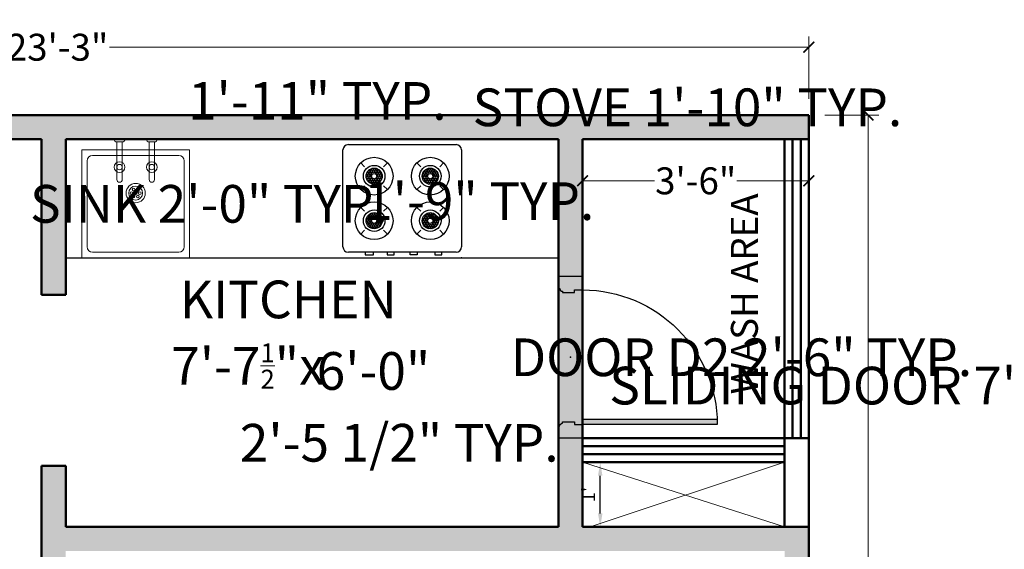
# Model space of a CAD drawing. Units: inches. Extents: x 4508 to 5907, y 877 to 1592.
# Tile 18 of 20: x 5383 to 5566, y 1494 to 1592. Entities that reach past the tile are written whole.
import ezdxf

# ---------------------------------------------------------------- set-up
doc = ezdxf.new("R2010")
doc.units = ezdxf.units.IN
doc.layers.get('DEFPOINTS').update_dxf_attribs({"color": 8})
for name, color, linetype, lineweight in [('A-ANNO-DIMS', 2, 'Continuous', 18), ('A-ANNO-TEXT', 7, 'Continuous', 25), ('A-DOOR', 4, 'Continuous', 25), ('A-FLOR-CASE', 30, 'Continuous', 25), ('A-FLOR-FIXT', 8, 'Continuous', 18), ('A-FLOR-SHFT', 8, 'Continuous', 18), ('A-WALL', 7, 'Continuous', 50), ('A-WALL-PATT', 8, 'Continuous', 13)]:
    doc.layers.add(name, color=color, linetype=linetype, lineweight=lineweight)
doc.layers.add('doors & windows', color=30, linetype='Continuous')
doc.layers.add('furniture', color=24, linetype='Continuous')
doc.styles.get("Standard").update_dxf_attribs({"font": 'arial.ttf'})
doc.dimstyles.new('details', dxfattribs={"dimtxt": 5, "dimasz": 2, "dimexe": 2, "dimexo": 3, "dimgap": 1, "dimtad": 0, "dimdec": 1, "dimzin": 0, "dimdsep": 46, "dimlunit": 4, "dimtxsty": 'Standard', "dimblk": 'ARCHTICK', "dimcen": 3, "dimclrd": 256, "dimclre": 256, "dimclrt": 256, "dimadec": 0, "dimazin": 0, "dimtfac": 0.5, "dimtdec": 1, "dimtofl": 0, "dimtmove": 0, "dimatfit": 3, "dimldrblk": 'CLOSEDBLANK', "dimfxl": 2, "dimtolj": 1, "dimtzin": 0, "dimlwd": -1, "dimlwe": -1, "dimarcsym": 0})
doc.dimstyles.new('ISO-25', dxfattribs={"dimtxt": 2.5, "dimasz": 2.5, "dimexe": 1.25, "dimexo": 0.625, "dimtad": 1, "dimdec": 0, "dimlunit": 4, "dimtxsty": 'Standard', "dimcen": 2.5, "dimadec": 0, "dimazin": 0, "dimtfac": 1, "dimtdec": 0, "dimtmove": 0, "dimatfit": 3, "dimfxl": 1, "dimarcsym": 0})
doc.dimstyles.new('text', dxfattribs={"dimtxt": 7, "dimasz": 0, "dimexe": 3, "dimexo": 3, "dimgap": 0, "dimtad": 1, "dimtih": 1, "dimtoh": 1, "dimzin": 3, "dimdsep": 46, "dimlunit": 4, "dimtxsty": 'Standard', "dimblk": 'CLOSEDBLANK', "dimcen": 3, "dimse1": 1, "dimse2": 1, "dimsd1": 1, "dimsd2": 1, "dimclrd": 256, "dimclre": 256, "dimclrt": 256, "dimadec": 0, "dimazin": 0, "dimtfac": 0.5, "dimtofl": 0, "dimtmove": 0, "dimatfit": 3, "dimfxl": 3, "dimtolj": 1, "dimtzin": 0, "dimlwd": -1, "dimlwe": -1, "dimarcsym": 0})

# ---------------------------------------------------------------- blocks, each defined once
blk = doc.blocks.new('*D78')
at = {"layer": 'DEFPOINTS', "color": 0, "transparency": 16777216}
for p in [(5391.9, 1545.16), (5483.4, 1536.45), (5483.4, 1523.93)]:
    blk.add_point(p, dxfattribs=at)
at = {"layer": 'A-ANNO-DIMS', "color": 0, "transparency": 16777216, "insert": (5425.76, 1533.92), "char_height": 7, "attachment_point": 5}
blk.add_mtext('\\A1;       KITCHEN\\P7\'-7{\\H0.5x;\\S1/2;}"x', dxfattribs=at)
blk = doc.blocks.new('_ClosedBlank')
at = {"color": 0, "lineweight": -2}
for p, q in [((-1, 0.167), (0, 0)), ((-1, 0.167), (-1, -0.167)), ((0, 0), (-1, -0.167))]:
    blk.add_line(p, q, dxfattribs=at)
blk = doc.blocks.new('*D79')
at = {"layer": 'DEFPOINTS', "color": 0, "transparency": 16777216}
for p in [(5431.17, 1570.2), (5449.06, 1570.2), (5421.9, 1498.2)]:
    blk.add_point(p, dxfattribs=at)
at = {"layer": 'A-ANNO-DIMS', "color": 0, "transparency": 16777216, "insert": (5449.06, 1527.16), "char_height": 7, "attachment_point": 5}
blk.add_mtext('\\A1;6\'-0"', dxfattribs=at)
blk = doc.blocks.new('stove')
at = {"layer": 'furniture'}
h = blk.add_hatch(dxfattribs=at)
h.set_pattern_fill('HEX', color=256, angle=180, style=0)
h.set_pattern_definition([(360, (22, 21.5), (1e-16, 0.2165064), [0.125, -0.25]), (120, (22, 21.5), (-0.1875, -0.1082532), [0.125, -0.25]), (60, (22.125, 21.5), (-0.1875, 0.1082532), [0.125, -0.25])])
h.paths.add_polyline_path([(5.36, 16.21, 1), (8.36, 16.21, 1)])
h.paths.add_polyline_path([(7.36, 16.21, -1), (6.36, 16.21, -1)], flags=16)
h = blk.add_hatch(dxfattribs=at)
h.set_pattern_fill('HEX', color=256, angle=180, style=0)
h.set_pattern_definition([(180, (2e-13, 21.5), (-1e-16, 0.2165064), [0.125, -0.25]), (60, (2e-13, 21.5), (0.1875, -0.1082532), [0.125, -0.25]), (120, (-0.125, 21.5), (0.1875, 0.1082532), [0.125, -0.25])])
h.paths.add_polyline_path([(13.64, 16.21, 1), (16.64, 16.21, 1)])
h.paths.add_polyline_path([(15.64, 16.21, -1), (14.64, 16.21, -1)], flags=16)
h = blk.add_hatch(dxfattribs=at)
h.set_pattern_fill('HEX', color=256, angle=180, style=0)
h.set_pattern_definition([(360, (22, 0.5), (-1e-16, -0.2165064), [0.125, -0.25]), (240, (22, 0.5), (-0.1875, 0.1082532), [0.125, -0.25]), (300, (22.125, 0.5), (-0.1875, -0.1082532), [0.125, -0.25])])
h.paths.add_polyline_path([(8.36, 5.79, 1), (5.36, 5.79, 1)])
h.paths.add_polyline_path([(6.36, 5.79, -1), (7.36, 5.79, -1)], flags=16)
h = blk.add_hatch(dxfattribs=at)
h.set_pattern_fill('HEX', color=256, angle=180, style=0)
h.set_pattern_definition([(180, (2e-13, 0.5), (1e-16, -0.2165064), [0.125, -0.25]), (300, (2e-13, 0.5), (0.1875, 0.1082532), [0.125, -0.25]), (240, (-0.125, 0.5), (0.1875, -0.1082532), [0.125, -0.25])])
h.paths.add_polyline_path([(16.64, 5.79, 1), (13.64, 5.79, 1)])
h.paths.add_polyline_path([(14.64, 5.79, -1), (15.64, 5.79, -1)], flags=16)
for p, q in [((2, 22), (20, 22)), ((1, 1), (1, 21)), ((21, 21), (21, 1)), ((4.39, 18.69), (5.1, 17.98)), ((8.63, 17.98), (9.34, 18.69)), ((13.37, 17.98), (12.66, 18.69)), ((17.61, 18.69), (16.9, 17.98)), ((1, 17.86), (0.5, 17.86)), ((0.5, 17.86), (0.5, 16.36)), ((0.5, 16.36), (1, 16.36)), ((0.5, 13.8), (0.5, 12.5)), ((1, 13.8), (0.5, 13.8)), ((4.39, 13.74), (5.1, 14.45)), ((8.63, 14.45), (9.34, 13.74)), ((13.37, 14.45), (12.66, 13.74)), ((17.61, 13.74), (16.9, 14.45)), ((0.5, 12.5), (1, 12.5)), ((0.5, 9.5), (1, 9.5)), ((0.5, 8.2), (0.5, 9.5)), ((1, 8.2), (0.5, 8.2)), ((4.39, 8.26), (5.1, 7.55)), ((8.63, 7.55), (9.34, 8.26)), ((13.37, 7.55), (12.66, 8.26)), ((17.61, 8.26), (16.9, 7.55)), ((0.5, 4.94), (0.5, 3.64)), ((1, 4.94), (0.5, 4.94)), ((4.39, 3.31), (5.1, 4.02)), ((8.63, 4.02), (9.34, 3.31)), ((13.37, 4.02), (12.66, 3.31)), ((17.61, 3.31), (16.9, 4.02)), ((0.5, 3.64), (1, 3.64)), ((20, 0), (2, 0))]:
    blk.add_line(p, q, dxfattribs=at)
for centre, radius in [((6.86, 16.21), 3.5), ((15.14, 16.21), 3.5), ((6.86, 16.21), 2), ((6.86, 16.21), 1.5), ((6.86, 16.21), 0.5), ((15.14, 16.21), 2), ((15.14, 16.21), 1.5), ((15.14, 16.21), 0.5), ((6.86, 5.79), 3.5), ((15.14, 5.79), 3.5), ((6.86, 5.79), 2), ((15.14, 5.79), 2), ((6.86, 5.79), 1.5), ((6.86, 5.79), 0.5), ((15.14, 5.79), 1.5), ((15.14, 5.79), 0.5)]:
    blk.add_circle(centre, radius, dxfattribs=at)
for centre, start, end in [((2, 21), 90, 180), ((20, 21), 0, 90), ((2, 1), 180, 270), ((20, 1), 270, 0)]:
    blk.add_arc(centre, 1, start, end, dxfattribs=at)
at = {"layer": 'furniture', "ltscale": 9}
blk.add_point((0, 0), dxfattribs=at)
blk = doc.blocks.new('sink')
for p, q in [((0, 0), (-24, 0)), ((0, 0), (0, 0)), ((-22, -3), (-2, -3)), ((-22, -23), (-22, -3)), ((-2, -3), (-2, -23)), ((-21, -21), (-21, -5)), ((-20, -4), (-4, -4)), ((-3, -5), (-3, -21)), ((0, -9), (0, -11)), ((-0.5, -9.5), (-7.5, -9.5)), ((-0.5, -10.5), (-7.5, -10.5)), ((-0.5, -9.5), (-0.5, -10.5)), ((-0.5, -15.5), (-7.5, -15.5)), ((-0.5, -15.5), (-0.5, -16.5)), ((0, -15), (0, -17)), ((-0.5, -16.5), (-7.5, -16.5)), ((-22, -23), (-2, -23)), ((-20, -22), (-4, -22))]:
    blk.add_line(p, q)
for centre, radius in [((-5.18, -10), 1), ((-5.18, -10), 0.5), ((-10, -13), 1.79), ((-10, -13), 1.29), ((-10.66, -12.62), 0.25), ((-10, -12.24), 0.25), ((-10, -13), 0.25), ((-9.34, -12.62), 0.25), ((-10.66, -13.38), 0.25), ((-10, -13.76), 0.25), ((-9.34, -13.38), 0.25), ((-5.18, -16), 1), ((-5.18, -16), 0.5)]:
    blk.add_circle(centre, radius)
for centre, radius, start, end in [((-20, -5), 1, 90, 180), ((-4, -5), 1, 0, 90), ((0.01, -9.51), 0.511, 91.1728, 178.8272), ((-7.5, -10), 0.5, 90, 270), ((0.01, -10.49), 0.511, 181.1728, 268.8272), ((-7.5, -16), 0.5, 90, 270), ((0.01, -15.51), 0.511, 91.1728, 178.8272), ((0.01, -16.49), 0.511, 181.1728, 268.8272), ((-20, -21), 1, 180, 270), ((-4, -21), 1, 270, 0)]:
    blk.add_arc(centre, radius, start, end)
blk = doc.blocks.new('*D80')
at = {"layer": 'A-ANNO-DIMS', "color": 0, "lineweight": -2, "transparency": 16777216}
for p, q in [((5488.53, 1510.2), (5492.43, 1510.2)), ((5491.18, 1500.7), (5491.18, 1507.7)), ((5488.53, 1498.2), (5492.43, 1498.2))]:
    blk.add_line(p, q, dxfattribs=at)
at = {"layer": 'A-ANNO-DIMS', "color": 0, "transparency": 16777216}
for points in [[(5490.76, 1507.7), (5491.59, 1507.7), (5491.18, 1510.2)], [(5490.76, 1500.7), (5491.59, 1500.7), (5491.18, 1498.2)]]:
    blk.add_solid(points, dxfattribs=at)
at = {"layer": 'DEFPOINTS', "color": 0, "transparency": 16777216}
for p in [(5487.9, 1510.2), (5491.18, 1510.2), (5487.9, 1498.2)]:
    blk.add_point(p, dxfattribs=at)
at = {"layer": 'A-ANNO-DIMS', "color": 0, "transparency": 16777216, "insert": (5489.3, 1504.2), "char_height": 2.5, "attachment_point": 5, "rotation": 90}
blk.add_mtext("1'", dxfattribs=at)
blk = doc.blocks.new('D2')
at = {"layer": 'doors & windows'}
h = blk.add_hatch(dxfattribs=at)
h.set_pattern_fill('DOTS', color=256, scale=2, angle=180, style=0)
h.set_pattern_definition([(180, (0, -4), (-0.0625, -0.125), [0, -0.125])])
h.paths.add_polyline_path([(2.5, 0), (3.5, 0), (3.5, 24.98, 0.010003), (2.5, 25)])
h = blk.add_hatch(dxfattribs=at)
h.set_pattern_fill('DOTS', color=256, scale=2, angle=180, style=0)
h.set_pattern_definition([(180, (0, 0), (-0.0625, -0.125), [0, -0.125])])
edge = h.paths.add_edge_path()
edge.add_line((27.5, 0), (27.5, -1.5))
edge.add_line((27.5, -1.5), (27, -1.5))
edge.add_line((27, -1.5), (27, -3.75))
edge.add_line((27, -3.75), (27.25, -3.75))
edge.add_arc((27.76, -3.74), 0.509, 181.0059, 268.9941)
edge.add_line((27.75, -4.25), (27.75, -4.5))
edge.add_line((27.75, -4.5), (30, -4.5))
edge.add_line((30, -4.5), (30, 0))
edge.add_line((30, 0), (27.5, 0))
edge = h.paths.add_edge_path()
edge.add_line((2.5, -1.5), (2.5, 0))
edge.add_line((2.5, 0), (0, 0))
edge.add_line((0, 0), (0, -4.5))
edge.add_line((0, -4.5), (2.25, -4.5))
edge.add_line((2.25, -4.5), (2.25, -4.25))
edge.add_arc((2.24, -3.74), 0.509, 271.0059, 358.9941)
edge.add_line((2.75, -3.75), (3, -3.75))
edge.add_line((3, -3.75), (3, -1.5))
edge.add_line((3, -1.5), (2.5, -1.5))
for p, q in [((0, 0), (0, -4.5)), ((30, 0), (30, -4.5))]:
    blk.add_line(p, q)
blk.add_lwpolyline([(3.5, 0), (3.5, 25), (2.5, 25), (2.5, 0)], close=True, dxfattribs=at)
for points in [[(3, -3.75), (3, -1.5), (2.5, -1.5), (2.5, 0), (0, 0)], [(27, -3.75), (27, -1.5), (27.5, -1.5), (27.5, 0), (30, 0)], [(0, -4.5), (2.25, -4.5)], [(30, -4.5), (27.75, -4.5)]]:
    blk.add_lwpolyline(points, dxfattribs=at)
for points in [[(2.25, -4.5), (2.25, -4.25, 0.403966), (2.75, -3.75), (3, -3.75)], [(27.75, -4.5), (27.75, -4.25, -0.403966), (27.25, -3.75), (27, -3.75)]]:
    blk.add_lwpolyline(points, format="xyb", dxfattribs=at)
at = {"layer": 'doors & windows', "ltscale": 6}
blk.add_arc((2.5, 0), 25, 0, 90, dxfattribs=at)
at = {"layer": 'doors & windows'}
blk.add_point((15, -2.25), dxfattribs=at)
blk = doc.blocks.new('_ArchTick')
at = {"color": 0, "linetype": 'ByBlock', "const_width": 0.15}
blk.add_lwpolyline([(-0.5, -0.5), (0.5, 0.5)], dxfattribs=at)
blk = doc.blocks.new('*D81')
at = {"layer": 'A-ANNO-DIMS', "color": 0, "transparency": 16777216}
for p, q in [((5487.9, 1567.2), (5487.9, 1560.48)), ((5529.9, 1567.2), (5529.9, 1560.48)), ((5487.9, 1562.48), (5501.26, 1562.48)), ((5529.9, 1562.48), (5516.55, 1562.48))]:
    blk.add_line(p, q, dxfattribs=at)
at = {"layer": 'DEFPOINTS', "color": 0, "transparency": 16777216}
for p in [(5487.9, 1570.2), (5529.9, 1570.2), (5529.9, 1562.48)]:
    blk.add_point(p, dxfattribs=at)
at = {"layer": 'A-ANNO-DIMS', "color": 0, "transparency": 16777216, "xscale": 2, "yscale": 2, "zscale": 2, "rotation": 180}
blk.add_blockref('_ArchTick', (5487.9, 1562.48), dxfattribs=at)
at = {"layer": 'A-ANNO-DIMS', "color": 0, "transparency": 16777216, "xscale": 2, "yscale": 2, "zscale": 2}
blk.add_blockref('_ArchTick', (5529.9, 1562.48), dxfattribs=at)
at = {"layer": 'A-ANNO-DIMS', "color": 0, "transparency": 16777216, "insert": (5508.9, 1562.48), "char_height": 5, "attachment_point": 5}
blk.add_mtext('\\A1;3\'-6"', dxfattribs=at)
blk = doc.blocks.new('*D82')
at = {"layer": 'DEFPOINTS', "color": 0, "transparency": 16777216}
for p in [(5255.4, 1510.81), (5387.4, 1507.41), (5387.4, 1493.7)]:
    blk.add_point(p, dxfattribs=at)
at = {"layer": 'A-ANNO-DIMS', "color": 0, "transparency": 16777216, "insert": (5317.71, 1516.81), "char_height": 7, "width": 116.2892, "attachment_point": 5}
blk.add_mtext('\\A1;       HALL\\P11\'-0"x', dxfattribs=at)
blk = doc.blocks.new('*D112')
at = {"layer": 'A-ANNO-DIMS', "color": 0, "transparency": 16777216}
for p, q in [((5250.9, 1577.7), (5250.9, 1589.3)), ((5529.9, 1577.7), (5529.9, 1589.3)), ((5250.9, 1587.3), (5380.77, 1587.3)), ((5529.9, 1587.3), (5400.03, 1587.3))]:
    blk.add_line(p, q, dxfattribs=at)
at = {"layer": 'DEFPOINTS', "color": 0, "transparency": 16777216}
for p in [(5529.9, 1587.3), (5250.9, 1574.7), (5529.9, 1574.7)]:
    blk.add_point(p, dxfattribs=at)
at = {"layer": 'A-ANNO-DIMS', "color": 0, "transparency": 16777216, "xscale": 2, "yscale": 2, "zscale": 2, "rotation": 180}
blk.add_blockref('_ArchTick', (5250.9, 1587.3), dxfattribs=at)
at = {"layer": 'A-ANNO-DIMS', "color": 0, "transparency": 16777216, "xscale": 2, "yscale": 2, "zscale": 2}
blk.add_blockref('_ArchTick', (5529.9, 1587.3), dxfattribs=at)
at = {"layer": 'A-ANNO-DIMS', "color": 0, "transparency": 16777216, "insert": (5390.4, 1587.3), "char_height": 5, "attachment_point": 5}
blk.add_mtext('\\A1;23\'-3"', dxfattribs=at)
blk = doc.blocks.new('*D113')
at = {"layer": 'A-ANNO-DIMS', "color": 0, "transparency": 16777216}
for p, q in [((5532.9, 1574.7), (5542.92, 1574.7)), ((5540.92, 1574.7), (5540.92, 1255.95)), ((5540.92, 926.7), (5540.92, 1245.46)), ((5532.9, 926.7), (5542.92, 926.7))]:
    blk.add_line(p, q, dxfattribs=at)
at = {"layer": 'DEFPOINTS', "color": 0, "transparency": 16777216}
for p in [(5529.9, 1574.7), (5540.92, 1574.7), (5529.9, 926.7)]:
    blk.add_point(p, dxfattribs=at)
at = {"layer": 'A-ANNO-DIMS', "color": 0, "transparency": 16777216, "xscale": 2, "yscale": 2, "zscale": 2}
for p, rotation in [((5540.92, 1574.7), 90), ((5540.92, 926.7), 270)]:
    blk.add_blockref('_ArchTick', p, dxfattribs=dict(at, rotation=rotation))
at = {"layer": 'A-ANNO-DIMS', "color": 0, "transparency": 16777216, "insert": (5540.92, 1250.7), "char_height": 5, "attachment_point": 5, "rotation": 90}
blk.add_mtext("\\A1;54'", dxfattribs=at)
blk = doc.blocks.new('*D146')
at = {"layer": 'DEFPOINTS', "color": 0, "transparency": 16777216}
for p in [(5512.9, 1544.7), (5517.4, 1544.7), (5512.9, 1514.7)]:
    blk.add_point(p, dxfattribs=at)
at = {"layer": 'A-ANNO-DIMS', "transparency": 16777216, "insert": (5517.4, 1529.7), "char_height": 7, "attachment_point": 5}
blk.add_mtext('\\A1;DOOR D2 2\'-6" TYP.', dxfattribs=at)
blk = doc.blocks.new('*D147')
at = {"layer": 'DEFPOINTS', "color": 0, "transparency": 16777216}
for p in [(5483.4, 1514.7), (5512.9, 1514.7), (5512.9, 1510.2)]:
    blk.add_point(p, dxfattribs=at)
at = {"layer": 'A-ANNO-DIMS', "transparency": 16777216, "insert": (5453.85, 1513.82), "char_height": 7, "attachment_point": 5}
blk.add_mtext('\\A1;2\'-5 1/2" TYP.', dxfattribs=at)
blk = doc.blocks.new('*D150')
at = {"layer": 'DEFPOINTS', "color": 0, "transparency": 16777216}
for p in [(5583.45, 1533.42), (5667.45, 1533.42), (5667.45, 1520.82)]:
    blk.add_point(p, dxfattribs=at)
at = {"layer": 'A-ANNO-DIMS', "transparency": 16777216, "insert": (5537.21, 1524.44), "char_height": 7, "attachment_point": 5}
blk.add_mtext('\\A1;SLIDING DOOR 7\'-0"', dxfattribs=at)
blk = doc.blocks.new('*D162')
at = {"layer": 'DEFPOINTS', "color": 0, "transparency": 16777216}
for p in [(5443.4, 1572.5), (5443.4, 1569.2), (5465.4, 1569.2)]:
    blk.add_point(p, dxfattribs=at)
at = {"layer": 'A-ANNO-DIMS', "transparency": 16777216, "insert": (5507.37, 1576.13), "char_height": 7, "attachment_point": 5}
blk.add_mtext('\\A1;STOVE 1\'-10" TYP.', dxfattribs=at)
blk = doc.blocks.new('*D163')
at = {"layer": 'DEFPOINTS', "color": 0, "transparency": 16777216}
for p in [(5465.4, 1569.2), (5468.7, 1569.2), (5465.4, 1548.2)]:
    blk.add_point(p, dxfattribs=at)
at = {"layer": 'A-ANNO-DIMS', "transparency": 16777216, "insert": (5468.7, 1558.7), "char_height": 7, "attachment_point": 5}
blk.add_mtext('\\A1;1\'-9" TYP.', dxfattribs=at)
blk = doc.blocks.new('*D164')
at = {"layer": 'DEFPOINTS', "color": 0, "transparency": 16777216}
for p in [(5414.9, 1570.2), (5418.5, 1570.2), (5414.9, 1546.2)]:
    blk.add_point(p, dxfattribs=at)
at = {"layer": 'A-ANNO-DIMS', "transparency": 16777216, "insert": (5418.5, 1558.2), "char_height": 7, "attachment_point": 5}
blk.add_mtext('\\A1;SINK 2\'-0" TYP.', dxfattribs=at)
blk = doc.blocks.new('*D165')
at = {"layer": 'DEFPOINTS', "color": 0, "transparency": 16777216}
for p in [(5391.9, 1573.8), (5391.9, 1570.2), (5414.9, 1570.2)]:
    blk.add_point(p, dxfattribs=at)
at = {"layer": 'A-ANNO-DIMS', "transparency": 16777216, "insert": (5438.63, 1577.32), "char_height": 7, "attachment_point": 5}
blk.add_mtext('\\A1;1\'-11" TYP.', dxfattribs=at)
blk = doc.blocks.new('*D174')
at = {"layer": 'DEFPOINTS', "color": 0, "transparency": 16777216}
for p in [(5294.35, 1476.58), (5294.35, 1472.05), (5324.54, 1472.05)]:
    blk.add_point(p, dxfattribs=at)
at = {"layer": 'A-ANNO-DIMS', "transparency": 16777216, "insert": (5362.41, 1480.2), "char_height": 7, "attachment_point": 5}
blk.add_mtext('\\A1;CHAIR 2\'-6" TYP.', dxfattribs=at)

msp = doc.modelspace()

# ---------------------------------------------------------------- hatches: boundary and pattern name
at = {"layer": 'A-WALL-PATT'}
h = msp.add_hatch(color=256, dxfattribs=at)
h.dxf.hatch_style = 1
h.paths.add_polyline_path([(5529.903, 1303.204), (5388.02, 1303.204), (5388.02, 1294.204), (5391.903, 1294.204), (5391.903, 1205.704), (5396.403, 1205.704), (5396.403, 1294.204), (5489.403, 1294.204), (5489.403, 1256.139), (5493.903, 1256.139), (5493.903, 1294.204), (5529.903, 1294.204)], flags=17)
h.paths.add_polyline_path([(5346.02, 1303.204), (5322.903, 1303.204), (5322.903, 1321.388), (5313.903, 1321.388), (5313.903, 1303.204), (5259.903, 1303.204), (5259.903, 1381.204), (5313.903, 1381.204), (5313.903, 1359.674), (5322.903, 1359.674), (5322.903, 1381.204), (5338.979, 1381.204), (5338.979, 1390.204), (5331.903, 1390.204), (5331.903, 1442.704), (5255.403, 1442.704), (5255.403, 1570.204), (5387.403, 1570.204), (5387.403, 1541.271), (5391.903, 1541.271), (5391.903, 1570.204), (5483.403, 1570.204), (5483.403, 1498.204), (5391.903, 1498.204), (5391.903, 1509.559), (5387.403, 1509.559), (5387.403, 1390.204), (5380.979, 1390.204), (5380.979, 1381.204), (5387.403, 1381.204), (5529.903, 1381.204), (5529.903, 1498.204), (5487.903, 1498.204), (5487.903, 1570.204), (5529.903, 1570.204), (5529.903, 1574.704), (5250.903, 1574.704), (5250.903, 991.204), (5310.903, 991.204), (5310.903, 926.704), (5529.903, 926.704), (5529.903, 1210.204), (5525.403, 1210.204), (5525.403, 1103.704), (5499.903, 1103.704), (5499.903, 1210.204), (5493.903, 1210.204), (5493.903, 1256.139), (5489.403, 1256.139), (5489.403, 1210.204), (5461.584, 1210.204), (5461.584, 1205.704), (5495.403, 1205.704), (5495.403, 1103.704), (5436.903, 1103.704), (5436.903, 1051.204), (5391.954, 1051.204), (5391.954, 1103.03), (5391.954, 1107.53), (5255.403, 1108.204), (5255.403, 1294.204), (5346.02, 1294.204)])
h.paths.add_polyline_path([(5255.403, 1390.204), (5255.403, 1398.204), (5255.403, 1438.204), (5257.903, 1438.204), (5258.903, 1438.204), (5327.403, 1438.204), (5327.403, 1390.204), (5325.903, 1390.204)], flags=16)
h.paths.add_polyline_path([(5288.757, 1390.704), (5288.757, 1390.204), (5292.173, 1390.204), (5292.173, 1390.704)], flags=0)
h.paths.add_polyline_path([(5289.965, 1391.606), (5289.965, 1396.645), (5289.903, 1396.645), (5289.903, 1397.319), (5288.849, 1398.862), (5288.849, 1398.8), (5288.983, 1398.748), (5288.983, 1399.204), (5289.091, 1399.204), (5292.081, 1399.204), (5292.081, 1398.665), (5291.946, 1398.665), (5291.027, 1397.319), (5291.027, 1396.645), (5290.965, 1396.645), (5290.965, 1391.606)], flags=0)
h.paths.add_polyline_path([(5288.849, 1399.069, 2.6374395), (5289.056, 1398.835), (5289.117, 1399.087, 0.9346155)], flags=0)
h.paths.add_polyline_path([(5290.061, 1398.665), (5290.061, 1399.204), (5290.038, 1398.975)], flags=0)
h.paths.add_polyline_path([(5291.946, 1398.934, -1), (5291.946, 1398.665)], flags=0)
h.paths.add_polyline_path([(5289.414, 1398.967), (5289.414, 1399.204), (5289.63, 1399.204), (5289.63, 1398.363), (5290.051, 1397.184), (5290.76, 1397.184), (5290.869, 1398.665), (5290.869, 1399.204), (5290.815, 1398.665), (5290.815, 1399.204), (5291.462, 1399.204), (5291.462, 1398.816), (5290.879, 1397.184), (5290.051, 1397.184)], flags=0)
h.paths.add_polyline_path([(5273.903, 1392.056), (5269.591, 1392.056, 0.0901028), (5265.544, 1392.842), (5265.511, 1392.034, -0.3516542), (5265.903, 1391.546, -1), (5264.903, 1391.546, -0.3042165), (5265.213, 1392.008), (5265.167, 1392.84, 0.0880132), (5261.215, 1392.056), (5256.903, 1392.056), (5256.903, 1398.704, -0.4142136), (5259.403, 1401.204), (5271.403, 1401.204, -0.4142136), (5273.903, 1398.704)], flags=0)
h.paths.add_polyline_path([(5263.726, 1395.073, -1), (5267.08, 1395.073, -1)], flags=0)
h.paths.add_polyline_path([(5264.434, 1395.073, -0.695521), (5265.153, 1395.073, -1.1408699), (5265.403, 1395.585, -0.7522125), (5265.403, 1396.25, 0.3674806)], flags=0)
h.paths.add_polyline_path([(5265.153, 1394.399, -1), (5265.653, 1394.399, -1)], flags=0)
h.paths.add_polyline_path([(5265.905, 1395.077, -1), (5266.405, 1395.077, -1)], flags=0)
h.paths.add_polyline_path([(5307.994, 1403.113, -1), (5307.994, 1417.295), (5318.794, 1417.295, -0.4142136), (5319.794, 1416.295), (5320.794, 1416.295, -0.4142136), (5321.794, 1417.295), (5324.903, 1417.295, -0.4142136), (5325.903, 1416.295), (5325.903, 1404.113, -0.4142136), (5324.903, 1403.113), (5321.794, 1403.113, -0.4142136), (5320.794, 1404.113), (5319.794, 1404.113, -0.4142136), (5318.794, 1403.113)], flags=0)
h.paths.add_polyline_path([(5307.836, 1405.113, -1), (5307.836, 1415.295), (5315.591, 1415.295, -0.4142136), (5317.532, 1413.353), (5317.532, 1407.054, -0.4142136), (5315.591, 1405.113)], flags=0)
h.paths.add_polyline_path([(5312.032, 1408.204, -1), (5312.032, 1412.204), (5315.032, 1412.204, -0.4142136), (5316.032, 1411.204), (5316.032, 1409.204, -0.4142136), (5315.032, 1408.204)], flags=0)
h.paths.add_polyline_path([(5391.903, 1385.704), (5391.903, 1493.704), (5525.403, 1493.704), (5525.403, 1385.704)], flags=16)
h.paths.add_polyline_path([(5422.641, 1390.704), (5422.641, 1465.704, -0.9426302), (5422.641, 1467.704), (5494.547, 1467.704, -1), (5494.665, 1465.704), (5494.665, 1390.704, -0.9426302), (5494.665, 1388.704), (5422.759, 1388.704, -1)], flags=0)
h.paths.add_polyline_path([(5427.52, 1395.749, -0.0238564), (5427.614, 1403.949, 0.0884332), (5427.476, 1405.056, 0.0506693), (5427.273, 1405.463, -0.8716827), (5427.713, 1405.835, 0.0268855), (5431.815, 1405.361, 0.0306964), (5436.289, 1405.361, -0.0263641), (5445.798, 1405.259, 0.075811), (5450.408, 1405.53, 0.0687062), (5454.457, 1405.903, -1.0086747), (5454.781, 1405.482, 0.0692081), (5454.389, 1400.959, -0.0519468), (5454.356, 1394.996, 0.1195012), (5454.627, 1392.895, 0.0143508), (5454.796, 1392.489, -0.6962059), (5454.42, 1392.118, 0.1574808), (5448.747, 1392.794, -0.025536), (5432.749, 1392.774, 0.0920085), (5427.781, 1392.048, -0.9384848), (5427.137, 1392.455, 0.0063894), (5427.314, 1392.79, 0.0472995)], flags=0)
h.paths.add_polyline_path([(5426.125, 1411.372, 0.0617649), (5428.641, 1412.201), (5428.641, 1465.704), (5488.665, 1465.704), (5488.665, 1412.363, 0.2363822), (5467.6, 1412.052, -0.2252042)], flags=0)
h.paths.add_polyline_path([(5391.903, 1490.204), (5391.903, 1491.204), (5422.903, 1491.204), (5422.903, 1490.204)], flags=0)
h.paths.add_polyline_path([(5462.545, 1392.771, 0.1270318), (5462.866, 1394.996, -0.0519468), (5462.832, 1400.959, 0.0692081), (5462.441, 1405.482, -1.0086747), (5462.765, 1405.903, 0.0857004), (5471.424, 1405.259, -0.0263641), (5480.932, 1405.361, 0.0306964), (5485.407, 1405.361, 0.0268855), (5489.509, 1405.835, -0.8716827), (5489.949, 1405.463, 0.0506693), (5489.746, 1405.056, 0.0884332), (5489.608, 1403.949, -0.0238564), (5489.702, 1395.749, 0.0472995), (5489.908, 1392.79, 0.0063894), (5490.085, 1392.455, -0.9384848), (5489.441, 1392.048, 0.0920085), (5484.473, 1392.774, -0.025536), (5468.475, 1392.794, 0.1574808), (5462.802, 1392.118, -0.6962059), (5462.426, 1392.489, 0.0100173), (5462.546, 1392.771)], flags=0)
h.paths.add_polyline_path([(5387.454, 1103.03), (5387.454, 1100.53), (5387.454, 1099.53), (5387.454, 995.03), (5387.454, 991.204), (5391.954, 991.204), (5391.954, 1046.704), (5525.403, 1046.704), (5525.403, 931.182), (5391.954, 930.53), (5391.954, 960.53), (5387.454, 960.53), (5387.454, 930.53), (5315.403, 930.53), (5315.403, 991.204), (5323.403, 991.204), (5387.454, 991.204), (5387.454, 995.03), (5255.403, 995.704), (5255.403, 1103.704)], flags=16)
h.paths.add_polyline_path([(5379.264, 1062.889), (5379.264, 1060.156), (5385.764, 1061.889, -0.4526903), (5385.764, 1059.889), (5379.264, 1059.889), (5379.264, 1055.156), (5385.764, 1056.889, -0.4526903), (5385.764, 1054.889), (5379.264, 1054.889), (5379.264, 1050.156), (5385.764, 1051.889, -0.4526903), (5385.764, 1049.889), (5379.264, 1049.889), (5379.264, 1010.156), (5385.764, 1011.889, -0.4526903), (5385.764, 1009.889), (5379.264, 1009.889), (5379.264, 1005.156), (5385.764, 1006.889, -0.4526903), (5385.764, 1004.889), (5379.264, 1004.889), (5379.264, 1000.156), (5385.764, 1001.889, -0.4526903), (5385.764, 999.889), (5378.264, 999.889), (5370.764, 997.889, -0.6674863), (5370.764, 999.889), (5377.264, 999.889), (5377.264, 1004.623), (5370.764, 1002.889, -0.6674863), (5370.764, 1004.889), (5377.264, 1004.889), (5377.264, 1009.623), (5370.764, 1007.889, -0.6674863), (5370.764, 1009.889), (5377.264, 1009.889), (5377.264, 1049.623), (5370.764, 1047.889, -0.6674863), (5370.764, 1049.889), (5377.264, 1049.889), (5377.264, 1054.623), (5370.764, 1052.889, -0.6674863), (5370.764, 1054.889), (5377.264, 1054.889), (5377.264, 1059.623), (5370.764, 1057.889, -0.6674863), (5370.764, 1059.889), (5377.264, 1059.889), (5377.264, 1062.889)], flags=0)
h.paths.add_polyline_path([(5287.641, 1000.704), (5359.665, 1000.704), (5359.665, 1018.212, 0.3202856), (5332.6, 1022.052, -0.246494), (5287.641, 1023.128)], flags=0)
h.paths.add_polyline_path([(5359.547, 1077.704, -1), (5359.665, 1075.704), (5353.665, 1075.704), (5353.665, 1063.704), (5293.641, 1063.704), (5293.641, 1075.704), (5287.759, 1075.704, -1), (5287.641, 1077.704)], flags=0)
h.paths.add_polyline_path([(5441.403, 1099.204), (5525.403, 1099.204), (5525.403, 1051.204), (5441.403, 1051.204), (5441.403, 1059.204)], flags=16)
h.paths.add_polyline_path([(5441.403, 1096.704), (5466.403, 1096.704), (5466.403, 1095.704), (5441.403, 1095.704)], flags=0)
h.paths.add_polyline_path([(5445.403, 1062.204), (5457.403, 1062.204, -0.4142136), (5459.903, 1059.704), (5459.903, 1053.056), (5455.591, 1053.056, 0.0901028), (5451.544, 1053.842), (5451.511, 1053.034, -0.3516542), (5451.903, 1052.546, -1), (5450.903, 1052.546, -0.3042165), (5451.213, 1053.008), (5451.167, 1053.84, 0.0880132), (5447.215, 1053.056), (5442.903, 1053.056), (5442.903, 1059.704, -0.4142136)], flags=0)
h.paths.add_polyline_path([(5453.08, 1056.073, -1), (5449.726, 1056.073, -1)], flags=0)
h.paths.add_polyline_path([(5292.713, 1015.835, 0.0268855), (5296.815, 1015.361, 0.0306964), (5301.289, 1015.361, -0.0263641), (5310.798, 1015.259, 0.075811), (5315.408, 1015.53, 0.0687062), (5319.457, 1015.903, -1.0086747), (5319.781, 1015.482, 0.0692081), (5319.389, 1010.959, -0.0519468), (5319.356, 1004.996, 0.1195012), (5319.627, 1002.895, 0.0143508), (5319.796, 1002.489, -0.6962059), (5319.42, 1002.118, 0.1574808), (5313.747, 1002.794, -0.025536), (5297.749, 1002.774, 0.0920085), (5292.781, 1002.048, -0.9384848), (5292.137, 1002.455, 0.0063894), (5292.314, 1002.79, 0.0472995), (5292.52, 1005.749, -0.0238564), (5292.614, 1013.949, 0.0884332), (5292.476, 1015.056, 0.0506693), (5292.273, 1015.463, -0.8716827)], flags=0)
h.paths.add_polyline_path([(5450.434, 1056.073, -0.695521), (5451.153, 1056.073, -1.1408699), (5451.403, 1056.585, -0.7522125), (5451.403, 1057.25, 0.3674806)], flags=0)
h.paths.add_polyline_path([(5327.765, 1015.903, 0.0857004), (5336.424, 1015.259, -0.0263641), (5345.932, 1015.361, 0.0306964), (5350.407, 1015.361, 0.0268855), (5354.509, 1015.835, -0.8716827), (5354.949, 1015.463, 0.0506693), (5354.746, 1015.056, 0.0884332), (5354.608, 1013.949, -0.0238564), (5354.702, 1005.749, 0.0472995), (5354.908, 1002.79, 0.0063894), (5355.085, 1002.455, -0.9384848), (5354.441, 1002.048, 0.0920085), (5349.473, 1002.774, -0.025536), (5333.475, 1002.794, 0.1574808), (5327.802, 1002.118, -0.6962059), (5327.426, 1002.489, 0.0100173), (5327.546, 1002.771), (5327.545, 1002.771, 0.1270318), (5327.866, 1004.996, -0.0519468), (5327.832, 1010.959, 0.0692081), (5327.441, 1015.482, -1.0086747)], flags=0)
h.paths.add_polyline_path([(5452.405, 1056.077, -1), (5451.905, 1056.077, -1)], flags=0)
h.paths.add_polyline_path([(5451.653, 1055.399, -1), (5451.153, 1055.399, -1)], flags=0)
h.paths.add_polyline_path([(5472.958, 1051.704), (5472.958, 1051.204), (5476.374, 1051.204), (5476.374, 1051.704)], flags=0)
h.paths.add_polyline_path([(5476.282, 1060.204), (5476.282, 1059.665), (5476.147, 1059.665), (5475.228, 1058.319), (5475.228, 1057.645), (5475.166, 1052.606), (5474.166, 1052.606), (5474.166, 1057.645), (5474.104, 1057.645), (5474.104, 1058.319), (5473.05, 1059.862), (5473.05, 1059.8), (5473.184, 1059.748), (5473.184, 1060.204), (5473.292, 1060.204)], flags=0)
h.paths.add_polyline_path([(5473.05, 1060.069, 2.6374395), (5473.257, 1059.835), (5473.318, 1060.087, 0.9346155)], flags=0)
h.paths.add_polyline_path([(5473.831, 1060.204), (5473.831, 1059.363), (5474.252, 1058.184), (5474.371, 1058.184), (5474.262, 1059.665), (5474.262, 1060.204)], flags=0)
h.paths.add_polyline_path([(5475.501, 1060.204), (5475.501, 1059.363), (5475.555, 1059.514), (5475.555, 1060.204)], flags=0)
h.paths.add_polyline_path([(5474.855, 1060.204), (5474.908, 1060.127), (5474.908, 1060.204), (5474.855, 1059.665)], flags=0)
h.paths.add_polyline_path([(5476.147, 1059.934, -1), (5476.147, 1059.665)], flags=0)
h.paths.add_polyline_path([(5474.693, 1060.204), (5475.178, 1059.511), (5475.178, 1060.204), (5475.285, 1059.934), (5475.285, 1060.204), (5475.178, 1059.665), (5475.178, 1060.204), (5475.07, 1059.665), (5475.07, 1060.204), (5474.962, 1059.665), (5474.962, 1060.204), (5474.693, 1059.306)], flags=0)
h.paths.add_polyline_path([(5474.747, 1060.204), (5474.37, 1059.45), (5474.37, 1060.204), (5474.424, 1060.096), (5474.424, 1060.204), (5474.747, 1059.665)], flags=0)
h.paths.add_polyline_path([(5476.04, 1059.665), (5476.04, 1060.204), (5476.094, 1059.665), (5476.094, 1060.204)], flags=0)
h.paths.add_polyline_path([(5505.994, 1082.295), (5516.794, 1082.295, -0.4142136), (5517.794, 1081.295), (5518.794, 1081.295, -0.4142136), (5519.794, 1082.295), (5522.903, 1082.295, -0.4142136), (5523.903, 1081.295), (5523.903, 1069.113, -0.4142136), (5522.903, 1068.113), (5519.794, 1068.113, -0.4142136), (5518.794, 1069.113), (5517.794, 1069.113, -0.4142136), (5516.794, 1068.113), (5505.994, 1068.113, -1)], flags=0)
h.paths.add_polyline_path([(5505.836, 1080.295), (5513.591, 1080.295, -0.4142136), (5515.532, 1078.353), (5515.532, 1072.054, -0.4142136), (5513.591, 1070.113), (5505.836, 1070.113, -1)], flags=0)
h.paths.add_polyline_path([(5520.403, 963.695), (5520.403, 1035.72), (5502.895, 1035.72, 0.3202856), (5499.055, 1008.654, -0.246494), (5497.978, 963.695)], flags=0)
h.paths.add_polyline_path([(5445.403, 1035.72), (5445.403, 1029.72), (5457.403, 1029.72), (5457.403, 969.695), (5445.403, 969.695), (5445.403, 963.814, -1), (5443.403, 963.695), (5443.403, 1035.602, -1)], flags=0)
h.paths.add_polyline_path([(5510.032, 1077.204), (5513.032, 1077.204, -0.4142136), (5514.032, 1076.204), (5514.032, 1074.204, -0.4142136), (5513.032, 1073.204), (5510.032, 1073.204, -1)], flags=0)
h.paths.add_polyline_path([(5317.255, 989.704), (5323.903, 989.704, -0.4142136), (5326.403, 987.204), (5326.403, 975.204, -0.4142136), (5323.903, 972.704), (5317.255, 972.704), (5317.255, 977.016, 0.0901028), (5318.041, 981.063), (5317.233, 981.096, -0.8964437), (5316.245, 981.204, -0.8220123), (5317.207, 981.394), (5318.04, 981.44, 0.0880132), (5317.255, 985.392)], flags=0)
h.paths.add_polyline_path([(5321.949, 981.204, -1), (5318.594, 981.204, -1)], flags=0)
h.paths.add_polyline_path([(5362.454, 988.03), (5387.454, 988.03), (5387.454, 990.53), (5391.954, 990.53), (5391.704, 988.289, -0.4090807), (5391.204, 987.78), (5391.204, 987.53), (5388.954, 987.53), (5388.954, 988.03), (5387.454, 988.03), (5387.454, 987.03), (5362.474, 987.03, 0.4025427), (5387.454, 963.03), (5388.954, 963.03), (5388.954, 963.53), (5391.195, 963.28, -0.4142136), (5391.704, 962.771), (5391.954, 960.53), (5391.954, 962.78), (5391.704, 962.78, 0.4090807), (5391.195, 963.28), (5388.954, 963.53), (5388.954, 963.03), (5387.454, 963.03, -0.4025427), (5362.474, 987.03), (5362.454, 987.03)], flags=0)
h.paths.add_polyline_path([(5321.285, 981.204, -0.6555366), (5320.522, 981.204, -1.1195284), (5320.275, 980.701, -1.3500746), (5320.279, 980.026, 0.3749463)], flags=0)
h.paths.add_polyline_path([(5320.022, 981.923, -1), (5320.522, 981.923, -1)], flags=0)
h.paths.add_polyline_path([(5319.348, 981.204, -1), (5319.848, 981.204, -1)], flags=0)
h.paths.add_polyline_path([(5507.157, 1030.662, -0.0238564), (5515.358, 1030.756, 0.0472995), (5518.317, 1030.962, 0.0063894), (5518.652, 1031.139, -0.9384848), (5519.059, 1030.495, 0.0920085), (5518.333, 1025.527, -0.025536), (5518.313, 1009.53, 0.1574808), (5518.989, 1003.857, -0.6962059), (5518.618, 1003.48, 0.0100173), (5518.335, 1003.601), (5518.335, 1003.6, 0.1270318), (5516.111, 1003.921, -0.0519468), (5510.148, 1003.887, 0.0692081), (5505.624, 1003.495, -1.0086747), (5505.204, 1003.819, 0.0857004), (5505.848, 1012.479, -0.0263641), (5505.746, 1021.987, 0.0306964), (5505.746, 1026.462, 0.0268855), (5505.272, 1030.563, -0.8716827), (5505.644, 1031.004, 0.0506693), (5506.051, 1030.801, 0.0884332)], flags=0)
h.paths.add_polyline_path([(5368.045, 945.621), (5378.845, 945.621, -0.4142136), (5379.845, 944.621), (5380.845, 944.621, -0.4142136), (5381.845, 945.621), (5384.954, 945.621, -0.4142136), (5385.954, 944.621), (5385.954, 932.439, -0.4142136), (5384.954, 931.439), (5381.845, 931.439, -0.4142136), (5380.845, 932.439), (5379.845, 932.439, -0.4142136), (5378.845, 931.439), (5368.045, 931.439, -1)], flags=0)
h.paths.add_polyline_path([(5327.31, 931.03), (5327.31, 930.53), (5330.726, 930.53), (5330.726, 931.03)], flags=0)
h.paths.add_polyline_path([(5330.634, 939.53), (5330.634, 938.991), (5330.499, 938.991), (5329.579, 937.645), (5329.579, 936.971), (5329.518, 936.971), (5329.518, 931.933), (5328.518, 931.933), (5328.518, 936.971), (5328.456, 936.971), (5328.456, 937.645), (5327.402, 939.189), (5327.402, 939.126), (5327.536, 939.074), (5327.536, 939.53), (5327.644, 939.53)], flags=0)
h.paths.add_polyline_path([(5327.402, 939.395, 2.6374395), (5327.609, 939.161), (5327.67, 939.414, 0.9346155)], flags=0)
h.paths.add_polyline_path([(5328.021, 939.142), (5328.021, 939.53), (5327.967, 939.53), (5327.967, 939.293)], flags=0)
h.paths.add_polyline_path([(5328.614, 939.53), (5328.614, 938.991), (5328.723, 937.51), (5329.313, 937.51), (5329.422, 938.991), (5329.422, 939.53), (5329.368, 938.991), (5329.368, 939.53)], flags=0)
h.paths.add_polyline_path([(5329.853, 939.53), (5329.853, 938.689), (5329.907, 938.84), (5329.907, 939.53)], flags=0)
h.paths.add_polyline_path([(5330.499, 939.261, -1), (5330.499, 938.991)], flags=0)
h.paths.add_polyline_path([(5367.887, 943.621), (5375.641, 943.621, -0.4142136), (5377.583, 941.68), (5377.583, 935.38, -0.4142136), (5375.641, 933.439), (5367.887, 933.439, -1)], flags=0)
h.paths.add_polyline_path([(5509.267, 947.14), (5509.267, 939.64), (5511.267, 932.14, -0.4526903), (5509.267, 932.14), (5509.267, 938.64), (5504.534, 938.64), (5506.267, 932.14, -0.4526903), (5504.267, 932.14), (5504.267, 938.64), (5499.534, 938.64), (5501.267, 932.14, -0.4526903), (5499.267, 932.14), (5499.267, 938.64), (5459.534, 938.64), (5461.267, 932.14, -0.4526903), (5459.267, 932.14), (5459.267, 938.64), (5454.534, 938.64), (5456.267, 932.14, -0.4526903), (5454.267, 932.14), (5454.267, 938.64), (5449.534, 938.64), (5451.267, 932.14, -0.4526903), (5449.267, 932.14), (5449.267, 939.64), (5447.267, 947.14, -0.3030853), (5448.267, 947.808), (5508.266, 947.808, -0.3032033)], flags=0)
h.paths.add_polyline_path([(5510.148, 995.444, -0.0519468), (5516.111, 995.41, 0.1195012), (5518.212, 995.681, 0.0143508), (5518.618, 995.851, -0.6962059), (5518.989, 995.474, 0.1574808), (5518.313, 989.801, -0.025536), (5518.333, 973.804, 0.0920085), (5519.059, 968.836, -0.9384848), (5518.652, 968.192, 0.0063894), (5518.317, 968.369, 0.0472995), (5515.358, 968.575, -0.0238564), (5507.157, 968.669, 0.0884332), (5506.051, 968.531, 0.0506693), (5505.644, 968.327, -0.8716827), (5505.272, 968.768, 0.0268855), (5505.746, 972.869, 0.0306964), (5505.746, 977.344, -0.0263641), (5505.848, 986.852, 0.075811), (5505.576, 991.462, 0.0687062), (5505.204, 995.512, -1.0086747), (5505.624, 995.836, 0.0692081)], flags=0)
h.paths.add_polyline_path([(5372.083, 940.53), (5375.083, 940.53, -0.4142136), (5376.083, 939.53), (5376.083, 937.53, -0.4142136), (5375.083, 936.53), (5372.083, 936.53, -1)], flags=0)
h.paths.add_polyline_path([(5409.258, 1465.643), (5487.738, 1465.643), (5487.738, 1492.394), (5409.258, 1492.394)], flags=8)
h.paths.add_polyline_path([(5463.574, 1465.103), (5486.546, 1465.103), (5486.546, 1479.528), (5463.574, 1479.528)], flags=8)
h.paths.add_polyline_path([(5248.665, 1406.171), (5299.981, 1406.171), (5299.981, 1432.34), (5248.665, 1432.34)], flags=9)
h.paths.add_polyline_path([(5287.471, 1405.121), (5310.443, 1405.121), (5310.443, 1419.546), (5287.471, 1419.546)], flags=8)
h.paths.add_polyline_path([(5371.637, 1047.927), (5371.637, 1010.764), (5377.841, 1010.764), (5377.841, 1047.927)], flags=8)
h.paths.add_polyline_path([(5324.882, 1074.869), (5347.854, 1074.869), (5347.854, 1089.294), (5324.882, 1089.294)], flags=8)
h.paths.add_polyline_path([(5262.863, 1074.665), (5351.123, 1074.665), (5351.123, 1100.833), (5262.863, 1100.833)], flags=8)
h.paths.add_polyline_path([(5307.238, 938.814), (5363.988, 938.814), (5363.988, 964.982), (5307.238, 964.982)], flags=24)
h.paths.add_polyline_path([(5348.837, 937.997), (5371.809, 937.997), (5371.809, 952.422), (5348.837, 952.422)], flags=8)
h.paths.add_polyline_path([(5432.497, 1066.695), (5489.247, 1066.695), (5489.247, 1092.863), (5432.497, 1092.863)], flags=24)
h.paths.add_polyline_path([(5473.52, 1065.943), (5496.492, 1065.943), (5496.492, 1080.368), (5473.52, 1080.368)], flags=8)
h.paths.add_polyline_path([(5451.783, 984.266), (5480.194, 984.266), (5480.194, 998.691), (5451.783, 998.691)], flags=8)
h.paths.add_polyline_path([(5392.211, 983.632), (5481.554, 983.632), (5481.554, 1010.383), (5392.211, 1010.383)], flags=8)
h.paths.add_polyline_path([(5497.304, 946.267), (5460.142, 946.267), (5460.142, 940.062), (5497.304, 940.062)], flags=8)

# ---------------------------------------------------------------- linework, layer by layer
at = {"layer": 'A-FLOR-CASE'}
msp.add_line((5391.903, 1548.204), (5483.403, 1548.204), dxfattribs=at)
at = {"layer": 'A-FLOR-SHFT'}
for p, q in [((5525.403, 1498.204), (5487.903, 1510.204)), ((5489.326, 1498.204), (5525.403, 1510.204))]:
    msp.add_line(p, q, dxfattribs=at)
at = {"layer": 'A-WALL'}
for p, q in [((5250.903, 1574.704), (5529.903, 1574.704)), ((5529.903, 1574.704), (5529.903, 926.704)), ((5255.403, 1570.204), (5387.403, 1570.204)), ((5387.403, 1570.204), (5387.403, 1541.271)), ((5391.903, 1570.204), (5483.403, 1570.204)), ((5391.903, 1570.204), (5391.903, 1541.271)), ((5483.403, 1570.204), (5483.403, 1498.204)), ((5487.903, 1570.204), (5487.903, 1498.204)), ((5487.903, 1570.204), (5529.903, 1570.204)), ((5525.403, 1570.204), (5525.403, 1514.704)), ((5526.903, 1570.204), (5526.903, 1514.704)), ((5528.403, 1570.204), (5528.403, 1514.704)), ((5391.903, 1541.271), (5387.403, 1541.271)), ((5487.903, 1514.704), (5529.903, 1514.704)), ((5525.403, 1514.704), (5525.403, 1498.204)), ((5487.903, 1513.204), (5525.403, 1513.204)), ((5487.903, 1511.704), (5525.403, 1511.704)), ((5391.903, 1509.559), (5387.403, 1509.559)), ((5387.403, 1509.559), (5387.403, 1390.204)), ((5391.903, 1509.559), (5391.903, 1498.204)), ((5487.903, 1510.204), (5525.403, 1510.204)), ((5391.903, 1498.204), (5483.403, 1498.204)), ((5487.903, 1498.204), (5529.903, 1498.204))]:
    msp.add_line(p, q, dxfattribs=at)

# ---------------------------------------------------------------- block references
at = {"layer": 'A-DOOR', "xscale": -1, "rotation": 270}
msp.add_blockref('D2', (5487.903, 1514.704), dxfattribs=at)
at = {"layer": 'A-FLOR-FIXT', "rotation": 90}
for name, p in [('sink', (5391.903, 1570.204)), ('stove', (5465.403, 1548.204))]:
    msp.add_blockref(name, p, dxfattribs=at)

# ---------------------------------------------------------------- texts
at = {"layer": 'A-ANNO-TEXT'}
msp.add_text('WASH AREA', height=5, rotation=90, dxfattribs=at).set_placement((5520.444, 1522.812))

# ---------------------------------------------------------------- dimensions: what is measured, and where the dimension line sits
at = {"layer": 'A-ANNO-DIMS'}
for base, p1, p2, angle, text, picture, middle in [((5443.403, 1572.504), (5465.403, 1569.204), (5443.403, 1569.204), 180, 'STOVE <> TYP.', '*D162', (5507.372, 1576.126)), ((5391.903, 1573.804), (5414.903, 1570.204), (5391.903, 1570.204), 180, '<> TYP.', '*D165', (5438.627, 1577.32)), ((5418.503, 1570.204), (5414.903, 1546.204), (5414.903, 1570.204), 90, 'SINK <> TYP.', '*D164', (5418.503, 1558.204)), ((5468.703, 1569.204), (5465.403, 1548.204), (5465.403, 1569.204), 90, '<> TYP.', '*D163', (5468.703, 1558.704)), ((5517.403, 1544.704), (5512.903, 1514.704), (5512.903, 1544.704), 90, 'DOOR D2 <> TYP.', '*D146', (5517.403, 1529.704)), ((5294.351, 1476.577), (5324.541, 1472.048), (5294.351, 1472.048), 180, 'CHAIR <> TYP.', '*D174', (5362.406, 1480.196))]:
    dim = msp.add_linear_dim(base=base, p1=p1, p2=p2, angle=angle, text=text, dimstyle='text', override={"dimdec": 1, "dimrnd": 0, "dimzin": 1, "dimlunit": 4, "dimfrac": 2}, dxfattribs=at)
    dim.commit()
    dim.dimension.update_dxf_attribs({"geometry": picture, "text_midpoint": middle})
dim = msp.add_linear_dim(base=(5529.903, 1587.304), p1=(5250.903, 1574.704), p2=(5529.903, 1574.704), dimstyle='details', override={"dimclrd": 0, "dimclre": 0, "dimclrt": 0}, dxfattribs=at)
dim.commit()
dim.dimension.update_dxf_attribs({"geometry": '*D112', "text_midpoint": (5390.403, 1587.304)})
for base, p1, p2, dimstyle, picture, middle in [((5540.921, 1574.704), (5529.903, 926.704), (5529.903, 1574.704), 'details', '*D113', (5540.921, 1250.704)), ((5491.178, 1510.204), (5487.903, 1498.204), (5487.903, 1510.204), 'ISO-25', '*D80', (5489.298, 1504.204))]:
    dim = msp.add_linear_dim(base=base, p1=p1, p2=p2, angle=90, dimstyle=dimstyle, override={"dimclrd": 0, "dimclre": 0, "dimclrt": 0}, dxfattribs=at)
    dim.commit()
    dim.dimension.update_dxf_attribs({"geometry": picture, "text_midpoint": middle})
dim = msp.add_linear_dim(base=(5449.056, 1570.204), p1=(5421.903, 1498.204), p2=(5431.167, 1570.204), angle=90, dimstyle='text', override={"dimtad": 0, "dimclrd": 0, "dimclre": 0, "dimclrt": 0}, dxfattribs=at)
dim.commit()
dim.dimension.update_dxf_attribs({"geometry": '*D79', "text_midpoint": (5449.056, 1527.163), "dimtype": 160})
dim = msp.add_linear_dim(base=(5529.903, 1562.483), p1=(5487.903, 1570.204), p2=(5529.903, 1570.204), dimstyle='details', override={"dimclrd": 0, "dimclre": 0, "dimclrt": 0}, dxfattribs=at)
dim.commit()
dim.dimension.update_dxf_attribs({"geometry": '*D81', "text_midpoint": (5508.903, 1562.483), "dimtype": 160})
for base, p1, p2, text, picture, middle in [((5483.403, 1523.933), (5391.903, 1545.156), (5483.403, 1536.454), '       KITCHEN\\P<>x', '*D78', (5425.757, 1523.933)), ((5387.403, 1507.406), (5255.403, 1510.807), (5387.403, 1493.704), '       HALL\\P<>x', '*D82', (5317.713, 1507.406))]:
    dim = msp.add_linear_dim(base=base, p1=p1, p2=p2, text=text, dimstyle='text', override={"dimclrd": 0, "dimclre": 0, "dimclrt": 0}, dxfattribs=at)
    dim.commit()
    dim.dimension.update_dxf_attribs({"geometry": picture, "text_midpoint": middle, "dimtype": 160})
for base, p1, p2, text, picture, middle in [((5667.45, 1520.817), (5583.45, 1533.417), (5667.45, 1533.417), 'SLIDING DOOR <>', '*D150', (5537.214, 1524.438)), ((5512.903, 1510.204), (5483.403, 1514.704), (5512.903, 1514.704), '<> TYP.', '*D147', (5453.854, 1513.823))]:
    dim = msp.add_linear_dim(base=base, p1=p1, p2=p2, text=text, dimstyle='text', override={"dimdec": 1, "dimrnd": 0, "dimzin": 1, "dimlunit": 4, "dimfrac": 2}, dxfattribs=at)
    dim.commit()
    dim.dimension.update_dxf_attribs({"geometry": picture, "text_midpoint": middle})

doc.saveas('drawing.dxf')
